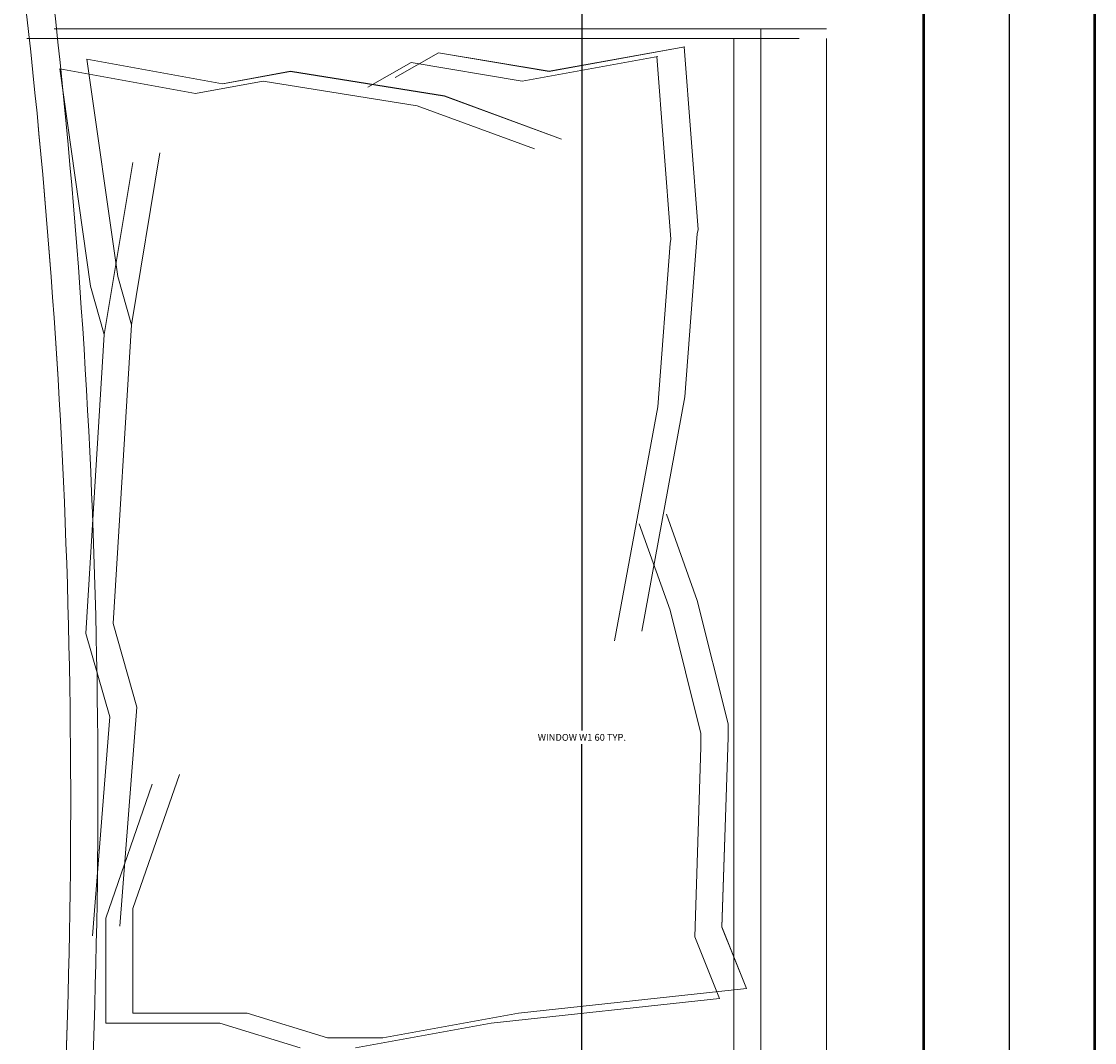
# Model space of a CAD drawing. Units: inches. Extents: x 1901 to 2863, y 888 to 2433.
# Tile 46 of 91: x 2725 to 2753, y 1595 to 1622. Entities that reach past the tile are written whole.
import ezdxf

# ---------------------------------------------------------------- set-up
doc = ezdxf.new("R2010")
doc.units = ezdxf.units.IN
for name, color, linetype, lineweight in [('A-ANNO-DIMS', 2, 'Continuous', 18), ('A-FURN', 8, 'Continuous', 18), ('A-GLAZ', 3, 'Continuous', 25), ('A-WALL', 7, 'Continuous', 50)]:
    doc.layers.add(name, color=color, linetype=linetype, lineweight=lineweight)
doc.styles.get("Standard").update_dxf_attribs({"font": 'arial.ttf'})
doc.dimstyles.get("Standard").update_dxf_attribs({"dimtxt": 0.18, "dimasz": 0.18, "dimexe": 0.18, "dimexo": 0.0625, "dimgap": 0.09, "dimtad": 0, "dimtih": 1, "dimtoh": 1, "dimdec": 4, "dimzin": 0, "dimdsep": 46, "dimtxsty": 'Standard', "dimcen": 0.09, "dimadec": 0, "dimazin": 0, "dimtfac": 1, "dimtdec": 4, "dimtofl": 0, "dimtmove": 0, "dimatfit": 3, "dimfxl": 1, "dimtolj": 1, "dimtzin": 0, "dimarcsym": 0})

# ---------------------------------------------------------------- blocks, each defined once
blk = doc.blocks.new('BED-DOUBLE')
for p, q in [((0.026, 57.778), (0.026, 4.122)), ((8.85, 30.041), (12.422, 30.69)), ((8.85, 30.041), (12.422, 30.69)), ((13.883, 30.69), (15.993, 30.041)), ((13.883, 30.69), (15.993, 30.041)), ((8.132, 29.785), (11.704, 30.434)), ((8.132, 29.784), (11.704, 30.434)), ((11.704, 30.434), (13.165, 30.434)), ((11.704, 30.434), (13.165, 30.434)), ((13.165, 30.434), (15.275, 29.785)), ((13.165, 30.434), (15.275, 29.784)), ((2.844, 29.392), (8.85, 30.041)), ((2.844, 29.392), (8.85, 30.041)), ((15.993, 30.041), (19.003, 30.041)), ((15.993, 30.041), (19.003, 30.041)), ((19.003, 30.041), (19.003, 27.282)), ((19.003, 30.041), (19.003, 27.282)), ((2.126, 29.136), (8.132, 29.785)), ((2.126, 29.135), (8.132, 29.784)), ((15.275, 29.785), (18.286, 29.785)), ((15.275, 29.784), (18.286, 29.784)), ((18.286, 29.785), (18.286, 27.026)), ((18.286, 29.784), (18.286, 27.025)), ((3.493, 27.769), (2.844, 29.392)), ((3.493, 27.769), (2.844, 29.392)), ((2.775, 27.513), (2.126, 29.136)), ((2.775, 27.512), (2.126, 29.135)), ((3.331, 22.777), (3.493, 27.769)), ((3.331, 22.778), (3.493, 27.769)), ((18.898, 21.983), (19.351, 27.745)), ((18.898, 21.983), (19.351, 27.745)), ((2.613, 22.521), (2.775, 27.513)), ((2.613, 22.521), (2.775, 27.512)), ((18.18, 21.727), (18.633, 27.489)), ((18.18, 21.727), (18.633, 27.488)), ((19.003, 27.282), (17.779, 23.752)), ((19.003, 27.282), (17.779, 23.751)), ((18.286, 27.026), (17.061, 23.495)), ((18.286, 27.025), (17.061, 23.495)), ((3.331, 22.417), (3.331, 22.778)), ((3.331, 22.416), (3.331, 22.777)), ((2.613, 22.16), (2.613, 22.521)), ((2.613, 22.16), (2.613, 22.521)), ((4.142, 19.171), (3.331, 22.417)), ((4.142, 19.17), (3.331, 22.416)), ((3.425, 18.914), (2.613, 22.16)), ((3.425, 18.914), (2.613, 22.16)), ((19.523, 19.782), (18.898, 21.983)), ((19.523, 19.782), (18.898, 21.983)), ((18.806, 19.526), (18.18, 21.727)), ((18.806, 19.526), (18.18, 21.727)), ((4.467, 13.815), (5.603, 19.982)), ((4.467, 13.814), (5.603, 19.982)), ((19.039, 11.912), (19.523, 19.782)), ((19.039, 11.912), (19.523, 19.782)), ((3.749, 13.558), (4.886, 19.726)), ((3.749, 13.558), (4.886, 19.725)), ((18.322, 11.656), (18.806, 19.526)), ((18.322, 11.655), (18.806, 19.526)), ((4.954, 16.898), (4.142, 19.171)), ((4.954, 16.898), (4.142, 19.17)), ((4.236, 16.642), (3.425, 18.914)), ((4.236, 16.642), (3.425, 18.914)), ((4.142, 9.522), (4.467, 13.815)), ((4.142, 9.522), (4.467, 13.814)), ((3.425, 9.265), (3.749, 13.558)), ((3.425, 9.265), (3.749, 13.558)), ((18.291, 7.385), (19.039, 11.912)), ((18.291, 7.385), (19.039, 11.912)), ((19.039, 11.912), (19.402, 10.639)), ((19.039, 11.912), (19.402, 10.64)), ((17.573, 7.129), (18.322, 11.656)), ((17.573, 7.128), (18.322, 11.655)), ((18.322, 11.656), (18.684, 10.383)), ((18.322, 11.655), (18.684, 10.383)), ((19.402, 10.64), (20.214, 4.917)), ((19.402, 10.639), (20.214, 4.917)), ((18.684, 10.383), (19.496, 4.661)), ((18.684, 10.383), (19.496, 4.661)), ((4.122, 9.403), (4.142, 9.522)), ((4.122, 9.404), (4.142, 9.522)), ((4.492, 4.597), (4.122, 9.404)), ((4.492, 4.597), (4.122, 9.403)), ((3.404, 9.147), (3.425, 9.265)), ((3.404, 9.147), (3.425, 9.265)), ((3.774, 4.341), (3.404, 9.147)), ((3.774, 4.341), (3.404, 9.147)), ((10.798, 5.891), (7.714, 7.027)), ((10.798, 5.891), (7.714, 7.027)), ((10.08, 5.635), (6.996, 6.771)), ((10.08, 5.634), (6.996, 6.771)), ((14.857, 5.242), (10.798, 5.891)), ((14.857, 5.242), (10.798, 5.891)), ((14.139, 4.986), (10.08, 5.635)), ((14.139, 4.985), (10.08, 5.634)), ((10.961, 4.755), (12.097, 5.404)), ((10.961, 4.755), (12.097, 5.404)), ((16.642, 5.567), (14.857, 5.242)), ((16.642, 5.566), (14.857, 5.242)), ((20.214, 4.917), (16.642, 5.567)), ((20.214, 4.917), (16.642, 5.566)), ((4.467, 4.592), (8.039, 5.242)), ((4.467, 4.593), (8.038, 5.242)), ((8.038, 5.242), (10.961, 4.755)), ((8.039, 5.242), (10.961, 4.755)), ((10.243, 4.498), (11.379, 5.148)), ((10.243, 4.499), (11.379, 5.148)), ((15.925, 5.31), (14.139, 4.985)), ((15.924, 5.31), (14.139, 4.986)), ((19.496, 4.661), (15.924, 5.31)), ((19.496, 4.661), (15.925, 5.31)), ((3.749, 4.336), (7.321, 4.986)), ((3.749, 4.336), (7.321, 4.985)), ((7.321, 4.986), (10.243, 4.499)), ((7.321, 4.985), (10.243, 4.498))]:
    blk.add_line(p, q)
for centre in [(205.143, 24.201), (205.143, 24.2), (204.426, 23.944), (204.426, 23.944)]:
    blk.add_arc(centre, 185.219, 176.08655, 186.78213)
blk = doc.blocks.new('WIN-60')
blk.add_line((0, 2.25), (60, 2.25))
blk = doc.blocks.new('*D19')
at = {"layer": 'A-ANNO-DIMS', "color": 0, "lineweight": -2, "transparency": 16777216}
for p, q in [((2748.364, 1633.499), (2739.246, 1633.499)), ((2739.426, 1633.319), (2739.426, 1603.682)), ((2739.426, 1573.679), (2739.426, 1603.316)), ((2748.364, 1573.499), (2739.246, 1573.499))]:
    blk.add_line(p, q, dxfattribs=at)
at = {"layer": 'A-ANNO-DIMS', "color": 0, "transparency": 16777216}
for points in [[(2739.396, 1633.319), (2739.456, 1633.319), (2739.426, 1633.499)], [(2739.396, 1573.679), (2739.456, 1573.679), (2739.426, 1573.499)]]:
    blk.add_solid(points, dxfattribs=at)
at = {"layer": 'Defpoints', "color": 0, "transparency": 16777216}
for p in [(2748.426, 1633.499), (2739.426, 1573.499), (2748.426, 1573.499)]:
    blk.add_point(p, dxfattribs=at)
at = {"layer": 'A-ANNO-DIMS', "color": 0, "transparency": 16777216, "insert": (2739.426, 1603.499), "char_height": 0.18, "attachment_point": 5}
blk.add_mtext('\\A1;WINDOW W1 60 TYP.', dxfattribs=at)

msp = doc.modelspace()

# ---------------------------------------------------------------- linework, layer by layer
at = {"layer": 'A-FURN'}
for p, q in [((2725.53, 1622.154), (2745.864, 1622.154)), ((2725.53, 1622.154), (2745.864, 1622.154)), ((2744.142, 1622.154), (2744.142, 1568.498)), ((2744.142, 1622.154), (2744.142, 1568.498)), ((2724.812, 1621.898), (2745.146, 1621.898)), ((2724.812, 1621.898), (2745.146, 1621.898)), ((2743.424, 1621.898), (2743.424, 1568.241)), ((2743.424, 1621.898), (2743.424, 1568.241))]:
    msp.add_line(p, q, dxfattribs=at)
at = {"layer": 'A-WALL'}
for p, q in [((2752.926, 1665.634), (2752.926, 1259.134)), ((2748.426, 1661.134), (2748.426, 1529.134))]:
    msp.add_line(p, q, dxfattribs=at)

# ---------------------------------------------------------------- block references
at = {"layer": 'A-FURN', "rotation": 180}
msp.add_blockref('BED-DOUBLE', (2745.89, 1626.019), dxfattribs=at)
at = {"layer": 'A-GLAZ', "rotation": 270.0000000000013}
msp.add_blockref('WIN-60', (2748.426, 1633.5), dxfattribs=at)

# ---------------------------------------------------------------- dimensions: what is measured, and where the dimension line sits
at = {"layer": 'A-ANNO-DIMS'}
dim = msp.add_linear_dim(base=(2739.426, 1573.499), p1=(2748.426, 1633.499), p2=(2748.426, 1573.499), angle=270, text='WINDOW W1 <> TYP.', dimstyle='Standard', override={"dimdec": 0, "dimlfac": 1, "dimrnd": 0, "dimzin": 0, "dimdsep": 46, "dimlunit": 2}, dxfattribs=at)
dim.commit()
dim.dimension.update_dxf_attribs({"geometry": '*D19', "text_midpoint": (2739.426, 1603.499)})

doc.saveas('drawing.dxf')
